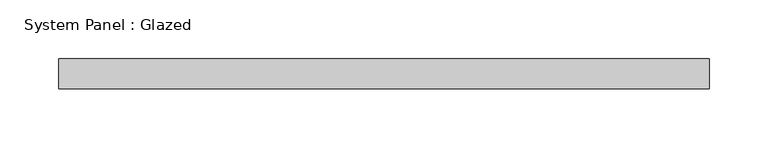
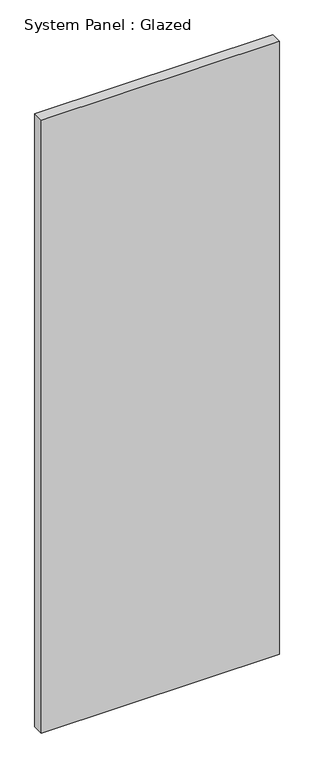
"""IFC4 building model written with IfcOpenShell, lengths in millimetres: plate geometry, System Panel : Glazed."""

from ifc_helpers import new_model, si_unit, origin, origin_with_axes, place, context, project, spatial, polyline, outline, extrude, source, transform, mapped, element, save


def system_panel_glazed_f147d628(model_context):
    return source(origin(), model_context, "Body", "SweptSolid", [
        extrude(outline(polyline([(276.225, 19.05), (-276.225, 19.05), (-276.225, 44.45), (276.225, 44.45), (276.225, 19.05)])), origin_with_axes(), (0.0, 0.0, 1.0), 1502.0255085),
    ])


if __name__ == "__main__":
    model = new_model("IFC4")
    model_context = context("Model", 3, world=origin())
    ifc_project = project(units=[si_unit("LENGTHUNIT", "METRE", prefix="MILLI")], contexts=[model_context])
    site = spatial("IfcSite", under=ifc_project)
    building = spatial("IfcBuilding", under=site)
    placement = place(None, origin())
    system_panel_glazed_shape = system_panel_glazed_f147d628(model_context)
    element("IfcPlate", 1, ObjectType="System Panel : Glazed", at=placement, inside=building, context=model_context, shape_type="MappedRepresentation", body=[
        mapped(system_panel_glazed_shape, transform((0.0, 0.0, 0.0), x_axis=(1.0, 0.0, 0.0), y_axis=(0.0, 1.0, 0.0), z_axis=(0.0, 0.0, 1.0))),
    ])
    save(model, "model.ifc")

# Revit data of these elements
# Type "System Panel : Glazed"
#   Construction Type Id = "GSP4R"
#   Analytic Construction = "1/8 in Pilkington single glazing"
#   Visual Light Transmittance = 0.9
#   Solar Heat Gain Coefficient = 0.86
#   Heat Transfer Coefficient (U) = 1.18115 BTU/(h·ft²·°F)
#   Define Thermal Properties by = 1
# Element 1 (IfcPlate, "System Panel : Glazed")
#   Materials on its faces: "Glass"
# Materials
#   "Glass": class "Glass", colour RGB 0 128 192, transparency 0.75, Description = "Soda Lime Glass", Cost = 0
